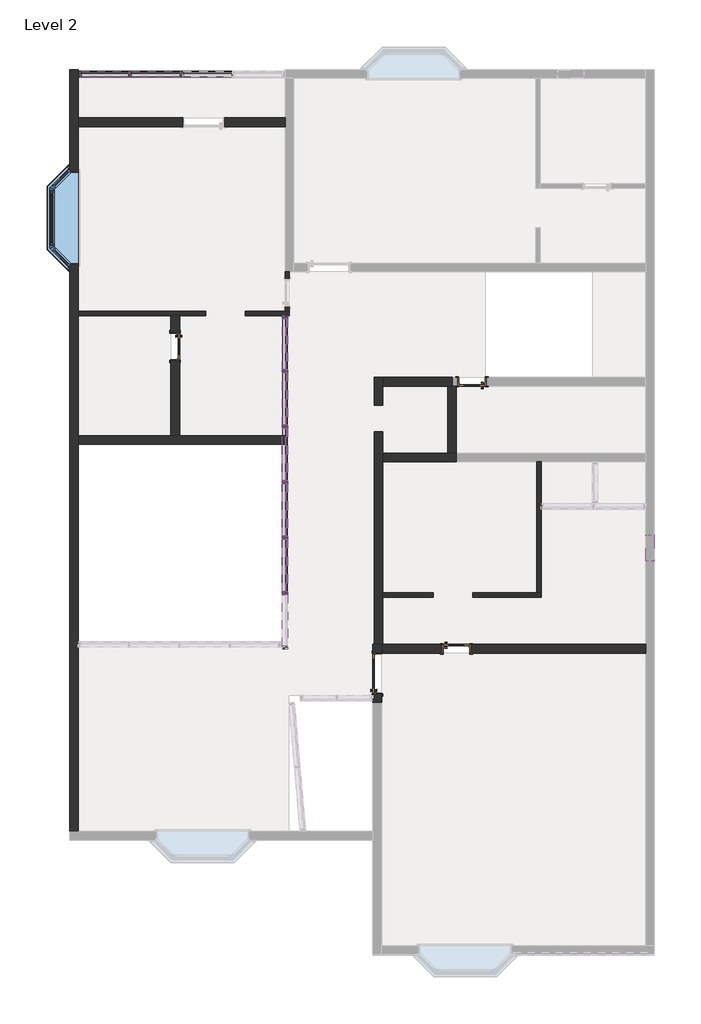
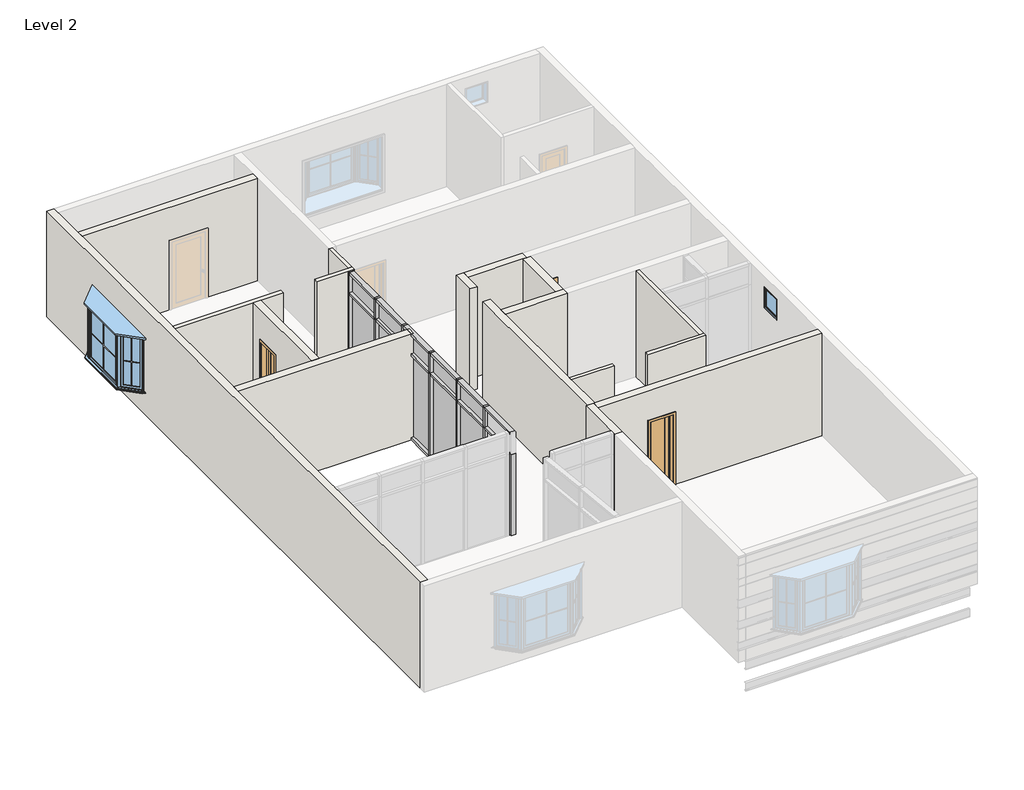
# One storey, part 4 of 5: 38 members, 17 walls, 12 plates, 4 doors, 2 windows.
"""IFC4 building model written with IfcOpenShell, lengths in millimetres."""

from ifc_helpers import new_model, si_unit, frame, origin, place, context, project, spatial, polyline, outline, extrude, faceted_brep, transform, mapped, element, save
from components import door_interior_single_1_panel_wood_5fe0af8f, door_interior_single_1_panel_wood_secondary_door_3_x_7_9c4ddfbd, member_6e77e263, member_47bfaf8a, member_f0fea5a5, member_ee409385, member_0e454ba5, member_3d117b0e, member_34cc32ae, member_667b8694, member_11eb1482, member_fb055d8d, member_66f4a397, member_e9262278, system_panel_glazed_d0e49211, system_panel_glazed_ecda40cd, system_panel_glazed_1bdee89b, system_panel_glazed_328a0544, system_panel_glazed_4fbe648e, system_panel_glazed_a20b732f, window_6846e476, window_9f89e8e4

model = new_model("IFC4")

# Units and contexts
model_context = context("Model", 3, world=origin())
ifc_project = project(units=[si_unit("LENGTHUNIT", "METRE", prefix="MILLI")], contexts=[model_context])

# Site, building, storey
site = spatial("IfcSite", under=ifc_project)
building = spatial("IfcBuilding", under=site)
storey = spatial("IfcBuildingStorey", under=building, Name="Level 2", Elevation=3048.0)

# Doors
placement = place(None, origin())
door_interior_single_1_panel_wood_shape = door_interior_single_1_panel_wood_5fe0af8f(model_context)
element("IfcDoor", 1, ObjectType="Door-Interior-Single-1_Panel-Wood", at=placement, inside=storey, context=model_context, shape_type="MappedRepresentation", body=[
    mapped(door_interior_single_1_panel_wood_shape, transform((-41818.5380314, -2936.7163973, 3048.0), x_axis=(1.0, 0.0, 0.0), y_axis=(0.0, 1.0, 0.0), z_axis=(0.0, 0.0, 1.0))),
])
element("IfcDoor", 2, ObjectType="Door-Interior-Single-1_Panel-Wood", at=placement, inside=storey, context=model_context, shape_type="MappedRepresentation", body=[
    mapped(door_interior_single_1_panel_wood_shape, transform((-41462.9380314, 3229.1336027, 3048.0), x_axis=(-1.0, 0.0, 0.0), y_axis=(0.0, -1.0, 0.0), z_axis=(0.0, 0.0, 1.0))),
])
element("IfcDoor", 3, ObjectType="Door-Interior-Single-1_Panel-Wood", at=placement, inside=storey, context=model_context, shape_type="MappedRepresentation", body=[
    mapped(door_interior_single_1_panel_wood_shape, transform((-48317.7630314, 4045.1086027, 3048.0), x_axis=(0.0, -1.0, 0.0), y_axis=(1.0, 0.0, 0.0), z_axis=(0.0, 0.0, 1.0))),
])
door_interior_single_1_panel_wood_secondary_door_3_x_7_shape = door_interior_single_1_panel_wood_secondary_door_3_x_7_9c4ddfbd(model_context)
element("IfcDoor", 4, ObjectType="Door-Interior-Single-1_Panel-Wood : SECONDARY DOOR 3' X 7'", at=placement, inside=storey, context=model_context, shape_type="MappedRepresentation", body=[
    mapped(door_interior_single_1_panel_wood_secondary_door_3_x_7_shape, transform((-43650.5130314, -3510.4922473, 3048.0), x_axis=(0.0, 1.0, 0.0), y_axis=(-1.0, 0.0, 0.0), z_axis=(0.0, 0.0, 1.0))),
])

# Members
member_shape = member_6e77e263(model_context)
element("IfcMember", 5, ObjectType="Rectangular Mullion : 2.5\" x 5\" rectangular", at=placement, inside=storey, context=model_context, shape_type="MappedRepresentation", body=[
    mapped(member_shape, transform((-45780.9380314, -1657.1913971, 5486.4), x_axis=(0.0, 1.0, 0.0), y_axis=(1.0, 0.0, 0.0), z_axis=(0.0, 0.0, -1.0))),
])
element("IfcMember", 6, ObjectType="Rectangular Mullion : 2.5\" x 5\" rectangular", at=placement, inside=storey, context=model_context, shape_type="MappedRepresentation", body=[
    mapped(member_shape, transform((-45780.9380314, -374.4913972, 5486.4), x_axis=(0.0, 1.0, 0.0), y_axis=(1.0, 0.0, 0.0), z_axis=(0.0, 0.0, -1.0))),
])
element("IfcMember", 7, ObjectType="Rectangular Mullion : 2.5\" x 5\" rectangular", at=placement, inside=storey, context=model_context, shape_type="MappedRepresentation", body=[
    mapped(member_shape, transform((-45780.9380314, 908.2086027, 5486.4), x_axis=(0.0, 1.0, 0.0), y_axis=(1.0, 0.0, 0.0), z_axis=(0.0, 0.0, -1.0))),
])
element("IfcMember", 8, ObjectType="Rectangular Mullion : 2.5\" x 5\" rectangular", at=placement, inside=storey, context=model_context, shape_type="MappedRepresentation", body=[
    mapped(member_shape, transform((-45780.9380314, 2190.9086026, 5486.4), x_axis=(0.0, 1.0, 0.0), y_axis=(1.0, 0.0, 0.0), z_axis=(0.0, 0.0, -1.0))),
])
element("IfcMember", 9, ObjectType="Rectangular Mullion : 2.5\" x 5\" rectangular", at=placement, inside=storey, context=model_context, shape_type="MappedRepresentation", body=[
    mapped(member_shape, transform((-45780.9380314, 3473.6086025, 5486.4), x_axis=(0.0, 1.0, 0.0), y_axis=(1.0, 0.0, 0.0), z_axis=(0.0, 0.0, -1.0))),
])
member_2_shape = member_47bfaf8a(model_context)
element("IfcMember", 10, ObjectType="Rectangular Mullion : 2.5\" x 5\" rectangular", at=placement, inside=storey, context=model_context, shape_type="MappedRepresentation", body=[
    mapped(member_2_shape, transform((-45780.9380314, 4756.3086027, 5486.4), x_axis=(0.0, 1.0, 0.0), y_axis=(1.0, 0.0, 0.0), z_axis=(0.0, 0.0, -1.0))),
])
member_3_shape = member_f0fea5a5(model_context)
element("IfcMember", 11, ObjectType="Rectangular Mullion : 2.5\" x 5\" rectangular", at=placement, inside=storey, context=model_context, shape_type="MappedRepresentation", body=[
    mapped(member_3_shape, transform((-45780.9380314, -1657.1913971, 3048.0), x_axis=(0.0, 1.0, 0.0), y_axis=(1.0, 0.0, 0.0), z_axis=(0.0, 0.0, -1.0))),
])
element("IfcMember", 12, ObjectType="Rectangular Mullion : 2.5\" x 5\" rectangular", at=placement, inside=storey, context=model_context, shape_type="MappedRepresentation", body=[
    mapped(member_3_shape, transform((-45780.9380314, -374.4913972, 3048.0), x_axis=(0.0, 1.0, 0.0), y_axis=(1.0, 0.0, 0.0), z_axis=(0.0, 0.0, -1.0))),
])
element("IfcMember", 13, ObjectType="Rectangular Mullion : 2.5\" x 5\" rectangular", at=placement, inside=storey, context=model_context, shape_type="MappedRepresentation", body=[
    mapped(member_3_shape, transform((-45780.9380314, 908.2086027, 3048.0), x_axis=(0.0, 1.0, 0.0), y_axis=(1.0, 0.0, 0.0), z_axis=(0.0, 0.0, -1.0))),
])
element("IfcMember", 14, ObjectType="Rectangular Mullion : 2.5\" x 5\" rectangular", at=placement, inside=storey, context=model_context, shape_type="MappedRepresentation", body=[
    mapped(member_3_shape, transform((-45780.9380314, 2190.9086026, 3048.0), x_axis=(0.0, 1.0, 0.0), y_axis=(1.0, 0.0, 0.0), z_axis=(0.0, 0.0, -1.0))),
])
element("IfcMember", 15, ObjectType="Rectangular Mullion : 2.5\" x 5\" rectangular", at=placement, inside=storey, context=model_context, shape_type="MappedRepresentation", body=[
    mapped(member_3_shape, transform((-45780.9380314, 3473.6086025, 3048.0), x_axis=(0.0, 1.0, 0.0), y_axis=(1.0, 0.0, 0.0), z_axis=(0.0, 0.0, -1.0))),
])
member_4_shape = member_ee409385(model_context)
element("IfcMember", 16, ObjectType="Rectangular Mullion : 2.5\" x 5\" rectangular", at=placement, inside=storey, context=model_context, shape_type="MappedRepresentation", body=[
    mapped(member_4_shape, transform((-45780.9380314, 4756.3086027, 3048.0), x_axis=(0.0, 1.0, 0.0), y_axis=(1.0, 0.0, 0.0), z_axis=(0.0, 0.0, -1.0))),
])
element("IfcMember", 17, ObjectType="Rectangular Mullion : 2.5\" x 5\" rectangular", at=placement, inside=storey, context=model_context, shape_type="MappedRepresentation", body=[
    mapped(member_4_shape, transform((-45780.9380314, -2939.8913973, 5486.4), x_axis=(0.0, -1.0, 0.0), y_axis=(1.0, 0.0, 0.0), z_axis=(0.0, 0.0, 1.0))),
])
member_5_shape = member_0e454ba5(model_context)
element("IfcMember", 18, ObjectType="Rectangular Mullion : 2.5\" x 5\" rectangular", at=placement, inside=storey, context=model_context, shape_type="MappedRepresentation", body=[
    mapped(member_5_shape, transform((-45780.9380314, 4692.8086027, 6096.0), x_axis=(0.0, 0.0, 1.0), y_axis=(1.0, 0.0, 0.0), z_axis=(0.0, 1.0, 0.0))),
])
element("IfcMember", 19, ObjectType="Rectangular Mullion : 2.5\" x 5\" rectangular", at=placement, inside=storey, context=model_context, shape_type="MappedRepresentation", body=[
    mapped(member_5_shape, transform((-45780.9380314, -1688.9413971, 6096.0), x_axis=(0.0, 0.0, 1.0), y_axis=(1.0, 0.0, 0.0), z_axis=(0.0, 1.0, 0.0))),
])
element("IfcMember", 20, ObjectType="Rectangular Mullion : 2.5\" x 5\" rectangular", at=placement, inside=storey, context=model_context, shape_type="MappedRepresentation", body=[
    mapped(member_5_shape, transform((-45780.9380314, 3505.3586025, 3048.0), x_axis=(0.0, 0.0, -1.0), y_axis=(1.0, 0.0, 0.0), z_axis=(0.0, -1.0, 0.0))),
])
member_6_shape = member_3d117b0e(model_context)
element("IfcMember", 21, ObjectType="Rectangular Mullion : 2.5\" x 5\" rectangular", at=placement, inside=storey, context=model_context, shape_type="MappedRepresentation", body=[
    mapped(member_6_shape, transform((-45780.9380314, -406.2413972, 6096.0), x_axis=(0.0, 0.0, 1.0), y_axis=(1.0, 0.0, 0.0), z_axis=(0.0, 1.0, 0.0))),
])
element("IfcMember", 22, ObjectType="Rectangular Mullion : 2.5\" x 5\" rectangular", at=placement, inside=storey, context=model_context, shape_type="MappedRepresentation", body=[
    mapped(member_6_shape, transform((-45780.9380314, 876.4586027, 6096.0), x_axis=(0.0, 0.0, 1.0), y_axis=(1.0, 0.0, 0.0), z_axis=(0.0, 1.0, 0.0))),
])
element("IfcMember", 23, ObjectType="Rectangular Mullion : 2.5\" x 5\" rectangular", at=placement, inside=storey, context=model_context, shape_type="MappedRepresentation", body=[
    mapped(member_6_shape, transform((-45780.9380314, 2159.1586026, 6096.0), x_axis=(0.0, 0.0, 1.0), y_axis=(1.0, 0.0, 0.0), z_axis=(0.0, 1.0, 0.0))),
])
element("IfcMember", 24, ObjectType="Rectangular Mullion : 2.5\" x 5\" rectangular", at=placement, inside=storey, context=model_context, shape_type="MappedRepresentation", body=[
    mapped(member_6_shape, transform((-45780.9380314, 3441.8586025, 6096.0), x_axis=(0.0, 0.0, 1.0), y_axis=(1.0, 0.0, 0.0), z_axis=(0.0, 1.0, 0.0))),
])
element("IfcMember", 25, ObjectType="Rectangular Mullion : 2.5\" x 5\" rectangular", at=placement, inside=storey, context=model_context, shape_type="MappedRepresentation", body=[
    mapped(member_6_shape, transform((-45780.9380314, -1625.4413971, 3048.0), x_axis=(0.0, 0.0, -1.0), y_axis=(1.0, 0.0, 0.0), z_axis=(0.0, -1.0, 0.0))),
])
element("IfcMember", 26, ObjectType="Rectangular Mullion : 2.5\" x 5\" rectangular", at=placement, inside=storey, context=model_context, shape_type="MappedRepresentation", body=[
    mapped(member_6_shape, transform((-45780.9380314, -342.7413972, 3048.0), x_axis=(0.0, 0.0, -1.0), y_axis=(1.0, 0.0, 0.0), z_axis=(0.0, -1.0, 0.0))),
])
element("IfcMember", 27, ObjectType="Rectangular Mullion : 2.5\" x 5\" rectangular", at=placement, inside=storey, context=model_context, shape_type="MappedRepresentation", body=[
    mapped(member_6_shape, transform((-45780.9380314, 939.9586027, 3048.0), x_axis=(0.0, 0.0, -1.0), y_axis=(1.0, 0.0, 0.0), z_axis=(0.0, -1.0, 0.0))),
])
element("IfcMember", 28, ObjectType="Rectangular Mullion : 2.5\" x 5\" rectangular", at=placement, inside=storey, context=model_context, shape_type="MappedRepresentation", body=[
    mapped(member_6_shape, transform((-45780.9380314, 2222.6586026, 3048.0), x_axis=(0.0, 0.0, -1.0), y_axis=(1.0, 0.0, 0.0), z_axis=(0.0, -1.0, 0.0))),
])
member_7_shape = member_34cc32ae(model_context)
element("IfcMember", 29, ObjectType="Rectangular Mullion : 2.5\" x 5\" rectangular", at=placement, inside=storey, context=model_context, shape_type="MappedRepresentation", body=[
    mapped(member_7_shape, transform((-45780.9380314, -1688.9413971, 5486.4), x_axis=(0.0, 0.0, 1.0), y_axis=(1.0, 0.0, 0.0), z_axis=(0.0, 1.0, 0.0))),
])
element("IfcMember", 30, ObjectType="Rectangular Mullion : 2.5\" x 5\" rectangular", at=placement, inside=storey, context=model_context, shape_type="MappedRepresentation", body=[
    mapped(member_7_shape, transform((-45780.9380314, 4692.8086027, 5486.4), x_axis=(0.0, 0.0, 1.0), y_axis=(1.0, 0.0, 0.0), z_axis=(0.0, 1.0, 0.0))),
])
member_8_shape = member_667b8694(model_context)
element("IfcMember", 31, ObjectType="Rectangular Mullion : 2.5\" x 5\" rectangular", at=placement, inside=storey, context=model_context, shape_type="MappedRepresentation", body=[
    mapped(member_8_shape, transform((-45780.9380314, -406.2413972, 5486.4), x_axis=(0.0, 0.0, 1.0), y_axis=(1.0, 0.0, 0.0), z_axis=(0.0, 1.0, 0.0))),
])
element("IfcMember", 32, ObjectType="Rectangular Mullion : 2.5\" x 5\" rectangular", at=placement, inside=storey, context=model_context, shape_type="MappedRepresentation", body=[
    mapped(member_8_shape, transform((-45780.9380314, 876.4586027, 5486.4), x_axis=(0.0, 0.0, 1.0), y_axis=(1.0, 0.0, 0.0), z_axis=(0.0, 1.0, 0.0))),
])
element("IfcMember", 33, ObjectType="Rectangular Mullion : 2.5\" x 5\" rectangular", at=placement, inside=storey, context=model_context, shape_type="MappedRepresentation", body=[
    mapped(member_8_shape, transform((-45780.9380314, 2159.1586026, 5486.4), x_axis=(0.0, 0.0, 1.0), y_axis=(1.0, 0.0, 0.0), z_axis=(0.0, 1.0, 0.0))),
])
element("IfcMember", 34, ObjectType="Rectangular Mullion : 2.5\" x 5\" rectangular", at=placement, inside=storey, context=model_context, shape_type="MappedRepresentation", body=[
    mapped(member_8_shape, transform((-45780.9380314, 3441.8586025, 5486.4), x_axis=(0.0, 0.0, 1.0), y_axis=(1.0, 0.0, 0.0), z_axis=(0.0, 1.0, 0.0))),
])
member_9_shape = member_11eb1482(model_context)
element("IfcMember", 35, ObjectType="Rectangular Mullion : 2.5\" x 5\" rectangular", at=placement, inside=storey, context=model_context, shape_type="MappedRepresentation", body=[
    mapped(member_9_shape, transform((-49394.0880313, 10344.3086027, 5209.4673659), x_axis=(0.0, 0.0, 1.0), y_axis=(0.0, -1.0, 0.0), z_axis=(1.0, 0.0, 0.0))),
])
member_10_shape = member_fb055d8d(model_context)
element("IfcMember", 36, ObjectType="Rectangular Mullion : 2.5\" x 5\" rectangular", at=placement, inside=storey, context=model_context, shape_type="MappedRepresentation", body=[
    mapped(member_10_shape, transform((-48200.2880314, 10344.3086027, 5209.4673659), x_axis=(0.0, 0.0, 1.0), y_axis=(0.0, -1.0, 0.0), z_axis=(1.0, 0.0, 0.0))),
])
element("IfcMember", 37, ObjectType="Rectangular Mullion : 2.5\" x 5\" rectangular", at=placement, inside=storey, context=model_context, shape_type="MappedRepresentation", body=[
    mapped(member_9_shape, transform((-50492.6380314, 10344.3086027, 3048.0), x_axis=(0.0, 0.0, -1.0), y_axis=(0.0, -1.0, 0.0), z_axis=(-1.0, 0.0, 0.0))),
])
element("IfcMember", 38, ObjectType="Rectangular Mullion : 2.5\" x 5\" rectangular", at=placement, inside=storey, context=model_context, shape_type="MappedRepresentation", body=[
    mapped(member_10_shape, transform((-49330.5880313, 10344.3086027, 3048.0), x_axis=(0.0, 0.0, -1.0), y_axis=(0.0, -1.0, 0.0), z_axis=(-1.0, 0.0, 0.0))),
])
element("IfcMember", 39, ObjectType="Rectangular Mullion : 2.5\" x 5\" rectangular", at=placement, inside=storey, context=model_context, shape_type="MappedRepresentation", body=[
    mapped(member_10_shape, transform((-48136.7880314, 10344.3086027, 3048.0), x_axis=(0.0, 0.0, -1.0), y_axis=(0.0, -1.0, 0.0), z_axis=(-1.0, 0.0, 0.0))),
])
member_11_shape = member_66f4a397(model_context)
element("IfcMember", 40, ObjectType="Rectangular Mullion : 2.5\" x 5\" rectangular", at=placement, inside=storey, context=model_context, shape_type="MappedRepresentation", body=[
    mapped(member_11_shape, transform((-49362.3380313, 10344.3086027, 3048.0), x_axis=(1.0, 0.0, 0.0), y_axis=(0.0, -1.0, 0.0), z_axis=(0.0, 0.0, -1.0))),
])
element("IfcMember", 41, ObjectType="Rectangular Mullion : 2.5\" x 5\" rectangular", at=placement, inside=storey, context=model_context, shape_type="MappedRepresentation", body=[
    mapped(member_11_shape, transform((-48168.5380314, 10344.3086027, 3048.0), x_axis=(1.0, 0.0, 0.0), y_axis=(0.0, -1.0, 0.0), z_axis=(0.0, 0.0, -1.0))),
])
member_12_shape = member_e9262278(model_context)
element("IfcMember", 42, ObjectType="Rectangular Mullion : 2.5\" x 5\" rectangular", at=placement, inside=storey, context=model_context, shape_type="MappedRepresentation", body=[
    mapped(member_12_shape, transform((-50556.1380314, 10344.3086027, 5209.4673659), x_axis=(-1.0, 0.0, 0.0), y_axis=(0.0, -1.0, 0.0), z_axis=(0.0, 0.0, 1.0))),
])

# Plates
system_panel_glazed_shape = system_panel_glazed_d0e49211(model_context)
element("IfcPlate", 43, ObjectType="System Panel : Glazed", at=placement, inside=storey, context=model_context, shape_type="MappedRepresentation", body=[
    mapped(system_panel_glazed_shape, transform((-45780.9380314, 4099.0836026, 3111.5), x_axis=(0.0, 1.0, 0.0), y_axis=(-1.0, 0.0, 0.0), z_axis=(0.0, 0.0, 1.0))),
])
system_panel_glazed_2_shape = system_panel_glazed_ecda40cd(model_context)
element("IfcPlate", 44, ObjectType="System Panel : Glazed", at=placement, inside=storey, context=model_context, shape_type="MappedRepresentation", body=[
    mapped(system_panel_glazed_2_shape, transform((-45780.9380314, -1015.8413971, 3111.5), x_axis=(0.0, 1.0, 0.0), y_axis=(-1.0, 0.0, 0.0), z_axis=(0.0, 0.0, 1.0))),
])
element("IfcPlate", 45, ObjectType="System Panel : Glazed", at=placement, inside=storey, context=model_context, shape_type="MappedRepresentation", body=[
    mapped(system_panel_glazed_2_shape, transform((-45780.9380314, 266.8586028, 3111.5), x_axis=(0.0, 1.0, 0.0), y_axis=(-1.0, 0.0, 0.0), z_axis=(0.0, 0.0, 1.0))),
])
element("IfcPlate", 46, ObjectType="System Panel : Glazed", at=placement, inside=storey, context=model_context, shape_type="MappedRepresentation", body=[
    mapped(system_panel_glazed_2_shape, transform((-45780.9380314, 1549.5586027, 3111.5), x_axis=(0.0, 1.0, 0.0), y_axis=(-1.0, 0.0, 0.0), z_axis=(0.0, 0.0, 1.0))),
])
element("IfcPlate", 47, ObjectType="System Panel : Glazed", at=placement, inside=storey, context=model_context, shape_type="MappedRepresentation", body=[
    mapped(system_panel_glazed_2_shape, transform((-45780.9380314, 2832.2586026, 3111.5), x_axis=(0.0, 1.0, 0.0), y_axis=(-1.0, 0.0, 0.0), z_axis=(0.0, 0.0, 1.0))),
])
system_panel_glazed_3_shape = system_panel_glazed_1bdee89b(model_context)
element("IfcPlate", 48, ObjectType="System Panel : Glazed", at=placement, inside=storey, context=model_context, shape_type="MappedRepresentation", body=[
    mapped(system_panel_glazed_3_shape, transform((-45780.9380314, 4099.0836026, 5518.15), x_axis=(0.0, 1.0, 0.0), y_axis=(-1.0, 0.0, 0.0), z_axis=(0.0, 0.0, 1.0))),
])
system_panel_glazed_4_shape = system_panel_glazed_328a0544(model_context)
element("IfcPlate", 49, ObjectType="System Panel : Glazed", at=placement, inside=storey, context=model_context, shape_type="MappedRepresentation", body=[
    mapped(system_panel_glazed_4_shape, transform((-45780.9380314, -1015.8413971, 5518.15), x_axis=(0.0, 1.0, 0.0), y_axis=(-1.0, 0.0, 0.0), z_axis=(0.0, 0.0, 1.0))),
])
element("IfcPlate", 50, ObjectType="System Panel : Glazed", at=placement, inside=storey, context=model_context, shape_type="MappedRepresentation", body=[
    mapped(system_panel_glazed_4_shape, transform((-45780.9380314, 266.8586028, 5518.15), x_axis=(0.0, 1.0, 0.0), y_axis=(-1.0, 0.0, 0.0), z_axis=(0.0, 0.0, 1.0))),
])
element("IfcPlate", 51, ObjectType="System Panel : Glazed", at=placement, inside=storey, context=model_context, shape_type="MappedRepresentation", body=[
    mapped(system_panel_glazed_4_shape, transform((-45780.9380314, 1549.5586027, 5518.15), x_axis=(0.0, 1.0, 0.0), y_axis=(-1.0, 0.0, 0.0), z_axis=(0.0, 0.0, 1.0))),
])
element("IfcPlate", 52, ObjectType="System Panel : Glazed", at=placement, inside=storey, context=model_context, shape_type="MappedRepresentation", body=[
    mapped(system_panel_glazed_4_shape, transform((-45780.9380314, 2832.2586026, 5518.15), x_axis=(0.0, 1.0, 0.0), y_axis=(-1.0, 0.0, 0.0), z_axis=(0.0, 0.0, 1.0))),
])
system_panel_glazed_5_shape = system_panel_glazed_4fbe648e(model_context)
element("IfcPlate", 53, ObjectType="System Panel : Glazed", at=placement, inside=storey, context=model_context, shape_type="MappedRepresentation", body=[
    mapped(system_panel_glazed_5_shape, transform((-49943.3630313, 10344.3086027, 3111.5), x_axis=(1.0, 0.0, 0.0), y_axis=(0.0, 1.0, 0.0), z_axis=(0.0, 0.0, 1.0))),
])
system_panel_glazed_6_shape = system_panel_glazed_a20b732f(model_context)
element("IfcPlate", 54, ObjectType="System Panel : Glazed", at=placement, inside=storey, context=model_context, shape_type="MappedRepresentation", body=[
    mapped(system_panel_glazed_6_shape, transform((-48765.4380313, 10344.3086027, 3111.5), x_axis=(1.0, 0.0, 0.0), y_axis=(0.0, 1.0, 0.0), z_axis=(0.0, 0.0, 1.0))),
])

# Walls
element("IfcWall", 55, ObjectType="INNER WALL 4\"", at=placement, inside=storey, context=model_context, shape_type="SweptSolid", body=[
    extrude(outline(polyline([(-42351.9380314, -1746.0913973), (-43520.3380314, -1746.0913973), (-43520.3380314, -1644.4913973), (-42351.9380314, -1644.4913973), (-42351.9380314, -1746.0913973)])), frame((0.0, 0.0, 3048.0), z_axis=(0.0, 0.0, 1.0), x_axis=(1.0, 0.0, 0.0)), (0.0, 0.0, 1.0), 3048.0),
])
element("IfcWall", 56, ObjectType="INNER WALL 4\"", at=placement, inside=storey, context=model_context, shape_type="Brep", body=[
    faceted_brep([(-41437.5380314, -1746.0913973, 3048.0), (-39862.7380314, -1746.0913973, 3048.0), (-39862.7380314, -1746.0913973, 6096.0), (-41437.5380314, -1746.0913973, 6096.0), (-41437.5380314, -1644.4913973, 3048.0), (-41437.5380314, -1644.4913973, 6096.0), (-39964.3380314, -1644.4913973, 6096.0), (-39862.7380314, -1644.4913973, 6096.0), (-39862.7380314, -1644.4913973, 3048.0), (-39964.3380314, -1644.4913973, 3048.0)], [[[0, 1, 2, 3]], [[4, 5, 6, 7, 8, 9]], [[1, 0, 4, 9, 8]], [[3, 2, 7, 6, 5]], [[0, 3, 5, 4]], [[2, 1, 8, 7]]]),
])
element("IfcWall", 57, ObjectType="INNER WALL 4\"", at=placement, inside=storey, context=model_context, shape_type="Brep", body=[
    faceted_brep([(-39862.7380314, -1644.4913973, 3048.0), (-39862.7380314, 303.5957124, 3048.0), (-39862.7380314, 354.3957124, 3048.0), (-39862.7380314, 1378.1086027, 3048.0), (-39862.7380314, 1378.1086027, 6096.0), (-39862.7380314, 354.3957124, 6096.0), (-39862.7380314, 303.5957124, 6096.0), (-39862.7380314, -1644.4913973, 6096.0), (-39964.3380314, -1644.4913973, 3048.0), (-39964.3380314, -1644.4913973, 6096.0), (-39964.3380314, 1378.1086027, 6096.0), (-39964.3380314, 1378.1086027, 3048.0)], [[[0, 1, 2, 3, 4, 5, 6, 7]], [[8, 9, 10, 11]], [[3, 2, 1, 0, 8, 11]], [[7, 6, 5, 4, 10, 9]], [[0, 7, 9, 8]], [[4, 3, 11, 10]]]),
])
element("IfcWall", 58, ObjectType="INNER WALL 4\"", at=placement, inside=storey, context=model_context, shape_type="Brep", body=[
    faceted_brep([(-50556.1380314, 4756.3086027, 3048.0), (-48422.5380314, 4756.3086027, 3048.0), (-48219.3380314, 4756.3086027, 3048.0), (-47609.7380314, 4756.3086027, 3048.0), (-47609.7380314, 4756.3086027, 6096.0), (-48219.3380314, 4756.3086027, 6096.0), (-48422.5380314, 4756.3086027, 6096.0), (-50556.1380314, 4756.3086027, 6096.0), (-50556.1380314, 4857.9086027, 3048.0), (-50556.1380314, 4857.9086027, 6096.0), (-47609.7380314, 4857.9086027, 6096.0), (-47609.7380314, 4857.9086027, 3048.0)], [[[0, 1, 2, 3, 4, 5, 6, 7]], [[8, 9, 10, 11]], [[3, 2, 1, 0, 8, 11]], [[4, 3, 11, 10]], [[7, 6, 5, 4, 10, 9]], [[0, 7, 9, 8]]]),
])
element("IfcWall", 59, ObjectType="INNER WALL 4\"", at=placement, inside=storey, context=model_context, shape_type="Brep", body=[
    faceted_brep([(-46695.3380314, 4756.3086027, 3048.0), (-45679.3380314, 4756.3086027, 3048.0), (-45679.3380314, 4756.3086027, 6096.0), (-46695.3380314, 4756.3086027, 6096.0), (-46695.3380314, 4857.9086027, 3048.0), (-46695.3380314, 4857.9086027, 6096.0), (-45780.9380314, 4857.9086027, 6096.0), (-45679.3380314, 4857.9086027, 6096.0), (-45679.3380314, 4857.9086027, 3048.0), (-45780.9380314, 4857.9086027, 3048.0)], [[[0, 1, 2, 3]], [[4, 5, 6, 7, 8, 9]], [[1, 0, 4, 9, 8]], [[3, 2, 7, 6, 5]], [[0, 3, 5, 4]], [[2, 1, 8, 7]]]),
])
element("IfcWall", 60, ObjectType="INNER WALL 4\"", at=placement, inside=storey, context=model_context, shape_type="SweptSolid", body=[
    extrude(outline(polyline([(4857.9086027, 6096.0), (5772.3086027, 6096.0), (5772.3086027, 3048.0), (5619.9086027, 3048.0), (5619.9086027, 5207.0), (4959.5086027, 5207.0), (4959.5086027, 3048.0), (4857.9086027, 3048.0), (4857.9086027, 6096.0)])), frame((-45780.9380314, 0.0, 0.0), z_axis=(1.0, 0.0, 0.0), x_axis=(0.0, 1.0, 0.0)), (0.0, 0.0, 1.0), 101.6),
])
element("IfcWall", 61, ObjectType="OUTER WALL 8\"", at=placement, inside=storey, context=model_context, shape_type="Brep", body=[
    faceted_brep([(-50759.3380314, 10445.9086027, 3048.0), (-50759.3380314, -7156.2913973, 3048.0), (-50759.3380314, -7156.2913973, 6096.0), (-50759.3380314, 10445.9086027, 6096.0), (-50759.3380314, 8133.1000114, 5232.4), (-50759.3380314, 5900.7171941, 5232.4), (-50759.3380314, 5900.7171941, 3657.6), (-50759.3380314, 8133.1000114, 3657.6), (-50556.1380314, 10445.9086027, 3048.0), (-50556.1380314, 10445.9086027, 5209.4673659), (-50556.1380314, 10445.9086027, 6096.0), (-50556.1380314, 10242.7086027, 6096.0), (-50556.1380314, 9328.3086027, 6096.0), (-50556.1380314, 9125.1086027, 6096.0), (-50556.1380314, 4857.9086027, 6096.0), (-50556.1380314, 4756.3086027, 6096.0), (-50556.1380314, 1987.7086027, 6096.0), (-50556.1380314, 1784.5086027, 6096.0), (-50556.1380314, -7156.2913973, 6096.0), (-50556.1380314, -7156.2913973, 3048.0), (-50556.1380314, 1784.5086027, 3048.0), (-50556.1380314, 1987.7086027, 3048.0), (-50556.1380314, 4756.3086027, 3048.0), (-50556.1380314, 4857.9086027, 3048.0), (-50556.1380314, 9125.1086027, 3048.0), (-50556.1380314, 9328.3086027, 3048.0), (-50556.1380314, 5950.1086027, 5232.4), (-50556.1380314, 8083.7086027, 5232.4), (-50556.1380314, 8083.7086027, 3657.6), (-50556.1380314, 5950.1086027, 3657.6), (-50709.9466227, 5950.1086027, 5232.4), (-50709.9466227, 8083.7086027, 5232.4), (-50709.9466227, 5950.1086027, 3657.6), (-50709.9466227, 8083.7086027, 3657.6)], [[[0, 1, 2, 3], [4, 5, 6, 7]], [[8, 9, 10, 11, 12, 13, 14, 15, 16, 17, 18, 19, 20, 21, 22, 23, 24, 25], [26, 27, 28, 29]], [[1, 0, 8, 25, 24, 23, 22, 21, 20, 19]], [[3, 2, 18, 17, 16, 15, 14, 13, 12, 11, 10]], [[2, 1, 19, 18]], [[0, 3, 10, 9, 8]], [[30, 5, 4, 31, 27, 26]], [[32, 29, 28, 33, 7, 6]], [[30, 26, 29, 32]], [[27, 31, 33, 28]], [[31, 4, 7, 33]], [[5, 30, 32, 6]]]),
])
element("IfcWall", 62, ObjectType="OUTER WALL 8\"", at=placement, inside=storey, context=model_context, shape_type="Brep", body=[
    faceted_brep([(-50556.1380314, 1784.5086027, 3048.0), (-45780.9380314, 1784.5086027, 3048.0), (-45780.9380314, 1784.5086027, 6096.0), (-50556.1380314, 1784.5086027, 6096.0), (-50556.1380314, 1987.7086027, 3048.0), (-50556.1380314, 1987.7086027, 6096.0), (-48422.5380314, 1987.7086027, 6096.0), (-48219.3380314, 1987.7086027, 6096.0), (-45780.9380314, 1987.7086027, 6096.0), (-45780.9380314, 1987.7086027, 3048.0), (-48219.3380314, 1987.7086027, 3048.0), (-48422.5380314, 1987.7086027, 3048.0)], [[[0, 1, 2, 3]], [[4, 5, 6, 7, 8, 9, 10, 11]], [[1, 0, 4, 11, 10, 9]], [[2, 1, 9, 8]], [[3, 2, 8, 7, 6, 5]], [[0, 3, 5, 4]]]),
])
element("IfcWall", 63, ObjectType="OUTER WALL 8\"", at=placement, inside=storey, context=model_context, shape_type="SweptSolid", body=[
    extrude(outline(polyline([(1987.7086027, 6096.0), (4756.3086027, 6096.0), (4756.3086027, 3048.0), (4375.3086027, 3048.0), (4375.3086027, 5207.0), (3714.9086027, 5207.0), (3714.9086027, 3048.0), (1987.7086027, 3048.0), (1987.7086027, 6096.0)])), frame((-48422.5380314, 0.0, 0.0), z_axis=(1.0, 0.0, 0.0), x_axis=(0.0, 1.0, 0.0)), (0.0, 0.0, 1.0), 203.2),
])
element("IfcWall", 64, ObjectType="OUTER WALL 8\"", at=placement, inside=storey, context=model_context, shape_type="Brep", body=[
    faceted_brep([(-43545.7380314, -2838.2913973, 6096.0), (-43545.7380314, -3041.4913973, 6096.0), (-43545.7380314, -4182.6930974, 6096.0), (-43545.7380314, -4182.6930974, 3048.0), (-43545.7380314, -3993.0922473, 3048.0), (-43545.7380314, -3993.0922473, 5207.0), (-43545.7380314, -3027.8922473, 5207.0), (-43545.7380314, -3027.8922473, 3048.0), (-43545.7380314, -2838.2913973, 3048.0), (-43748.9380314, -4182.6930974, 6096.0), (-43748.9380314, -2838.2913973, 6096.0), (-43748.9380314, -2838.2913973, 3048.0), (-43748.9380314, -3027.8922473, 3048.0), (-43748.9380314, -3027.8922473, 5207.0), (-43748.9380314, -3993.0922473, 5207.0), (-43748.9380314, -3993.0922473, 3048.0), (-43748.9380314, -4182.6930974, 3048.0), (-43723.5380314, -2838.2913973, 3048.0), (-43723.5380314, -2838.2913973, 6096.0)], [[[0, 1, 2, 3, 4, 5, 6, 7, 8]], [[9, 10, 11, 12, 13, 14, 15, 16]], [[11, 17, 8, 7, 12]], [[3, 16, 15, 4]], [[2, 1, 0, 18, 10, 9]], [[3, 2, 9, 16]], [[0, 8, 17, 11, 10, 18]], [[6, 13, 12, 7]], [[13, 6, 5, 14]], [[14, 5, 4, 15]]]),
])
element("IfcWall", 65, ObjectType="OUTER WALL 8\"", at=placement, inside=storey, context=model_context, shape_type="Brep", body=[
    faceted_brep([(-43545.7380314, -2838.2913973, 6096.0), (-43520.3380314, -2838.2913973, 6096.0), (-37449.7380314, -2838.2913973, 6096.0), (-37449.7380314, -2838.2913973, 3048.0), (-41488.3380314, -2838.2913973, 3048.0), (-41488.3380314, -2838.2913973, 5207.0), (-42148.7380314, -2838.2913973, 5207.0), (-42148.7380314, -2838.2913973, 3048.0), (-43520.3380314, -2838.2913973, 3048.0), (-43545.7380314, -2838.2913973, 3048.0), (-37449.7380314, -3041.4913973, 6096.0), (-43545.7380314, -3041.4913973, 6096.0), (-43545.7380314, -3041.4913973, 3048.0), (-42148.7380314, -3041.4913973, 3048.0), (-42148.7380314, -3041.4913973, 5207.0), (-41488.3380314, -3041.4913973, 5207.0), (-41488.3380314, -3041.4913973, 3048.0), (-37449.7380314, -3041.4913973, 3048.0)], [[[0, 1, 2, 3, 4, 5, 6, 7, 8, 9]], [[10, 11, 12, 13, 14, 15, 16, 17]], [[3, 17, 16, 4]], [[12, 9, 8, 7, 13]], [[2, 1, 0, 11, 10]], [[0, 9, 12, 11]], [[3, 2, 10, 17]], [[15, 5, 4, 16]], [[5, 15, 14, 6]], [[6, 14, 13, 7]]]),
])
element("IfcWall", 66, ObjectType="OUTER WALL 8\"", at=placement, inside=storey, context=model_context, shape_type="Brep", body=[
    faceted_brep([(-43520.3380314, -2838.2913973, 3048.0), (-43520.3380314, -1746.0913973, 3048.0), (-43520.3380314, -1644.4913973, 3048.0), (-43520.3380314, 1378.1086027, 3048.0), (-43520.3380314, 1581.3086027, 3048.0), (-43520.3380314, 2076.6086027, 3048.0), (-43520.3380314, 2076.6086027, 6096.0), (-43520.3380314, 1581.3086027, 6096.0), (-43520.3380314, 1378.1086027, 6096.0), (-43520.3380314, -1644.4913973, 6096.0), (-43520.3380314, -1746.0913973, 6096.0), (-43520.3380314, -2838.2913973, 6096.0), (-43723.5380314, -2838.2913973, 3048.0), (-43723.5380314, -2838.2913973, 6096.0), (-43723.5380314, 2076.6086027, 6096.0), (-43723.5380314, 2076.6086027, 3048.0), (-43545.7380314, -2838.2913973, 3048.0), (-43545.7380314, -2838.2913973, 6096.0)], [[[0, 1, 2, 3, 4, 5, 6, 7, 8, 9, 10, 11]], [[12, 13, 14, 15]], [[5, 4, 3, 2, 1, 0, 16, 12, 15]], [[6, 5, 15, 14]], [[11, 10, 9, 8, 7, 6, 14, 13, 17]], [[0, 11, 17, 13, 12, 16]]]),
])
element("IfcWall", 67, ObjectType="OUTER WALL 8\"", at=placement, inside=storey, context=model_context, shape_type="SweptSolid", body=[
    extrude(outline(polyline([(6096.0, -45780.9380314), (6096.0, -50556.1380314), (3048.0, -50556.1380314), (3048.0, -48143.1380314), (5105.4, -48143.1380314), (5105.4, -47177.9380314), (3048.0, -47177.9380314), (3048.0, -45780.9380314), (6096.0, -45780.9380314)])), frame((0.0, 9125.1086027, 0.0), z_axis=(0.0, 1.0, 0.0), x_axis=(0.0, 0.0, 1.0)), (0.0, 0.0, 1.0), 203.2),
])
element("IfcWall", 68, ObjectType="OUTER WALL 8\"", at=placement, inside=storey, context=model_context, shape_type="Brep", body=[
    faceted_brep([(-43520.3380314, 2686.2086027, 3048.0), (-43520.3380314, 3130.7086027, 3048.0), (-43520.3380314, 3333.9086027, 3048.0), (-43520.3380314, 3333.9086027, 6096.0), (-43520.3380314, 3130.7086027, 6096.0), (-43520.3380314, 2686.2086027, 6096.0), (-43723.5380314, 2686.2086027, 3048.0), (-43723.5380314, 2686.2086027, 6096.0), (-43723.5380314, 3333.9086027, 6096.0), (-43723.5380314, 3333.9086027, 3048.0)], [[[0, 1, 2, 3, 4, 5]], [[6, 7, 8, 9]], [[2, 1, 0, 6, 9]], [[5, 4, 3, 8, 7]], [[0, 5, 7, 6]], [[3, 2, 9, 8]]]),
])
element("IfcWall", 69, ObjectType="OUTER WALL 8\"", at=placement, inside=storey, context=model_context, shape_type="Brep", body=[
    faceted_brep([(-43520.3380314, 3130.7086027, 3048.0), (-42021.7380314, 3130.7086027, 3048.0), (-41920.1380314, 3130.7086027, 3048.0), (-41920.1380314, 3130.7086027, 6096.0), (-42021.7380314, 3130.7086027, 6096.0), (-43520.3380314, 3130.7086027, 6096.0), (-43520.3380314, 3333.9086027, 3048.0), (-43520.3380314, 3333.9086027, 6096.0), (-41920.1380314, 3333.9086027, 6096.0), (-41920.1380314, 3333.9086027, 3048.0)], [[[0, 1, 2, 3, 4, 5]], [[6, 7, 8, 9]], [[2, 1, 0, 6, 9]], [[3, 2, 9, 8]], [[5, 4, 3, 8, 7]], [[0, 5, 7, 6]]]),
])
element("IfcWall", 70, ObjectType="OUTER WALL 8\"", at=placement, inside=storey, context=model_context, shape_type="Brep", body=[
    faceted_brep([(-43520.3380314, 1378.1086027, 3048.0), (-41818.5380314, 1378.1086027, 3048.0), (-41818.5380314, 1378.1086027, 6096.0), (-43520.3380314, 1378.1086027, 6096.0), (-43520.3380314, 1581.3086027, 3048.0), (-43520.3380314, 1581.3086027, 6096.0), (-42021.7380314, 1581.3086027, 6096.0), (-41818.5380314, 1581.3086027, 6096.0), (-41818.5380314, 1581.3086027, 3048.0), (-42021.7380314, 1581.3086027, 3048.0)], [[[0, 1, 2, 3]], [[4, 5, 6, 7, 8, 9]], [[1, 0, 4, 9, 8]], [[3, 2, 7, 6, 5]], [[0, 3, 5, 4]], [[2, 1, 8, 7]]]),
])
element("IfcWall", 71, ObjectType="OUTER WALL 8\"", at=placement, inside=storey, context=model_context, shape_type="Brep", body=[
    faceted_brep([(-41818.5380314, 1581.3086027, 3048.0), (-41818.5380314, 3130.7086027, 3048.0), (-41818.5380314, 3130.7086027, 6096.0), (-41818.5380314, 1581.3086027, 6096.0), (-42021.7380314, 1581.3086027, 3048.0), (-42021.7380314, 1581.3086027, 6096.0), (-42021.7380314, 3130.7086027, 6096.0), (-42021.7380314, 3130.7086027, 3048.0), (-41920.1380314, 3130.7086027, 3048.0), (-41920.1380314, 3130.7086027, 6096.0)], [[[0, 1, 2, 3]], [[4, 5, 6, 7]], [[1, 0, 4, 7, 8]], [[3, 2, 9, 6, 5]], [[0, 3, 5, 4]], [[2, 1, 8, 7, 6, 9]]]),
])

# Windows
window_shape = window_6846e476(model_context)
element("IfcWindow", 72, ObjectType="Fixed : 24\" x 24\"", at=placement, inside=storey, context=model_context, shape_type="MappedRepresentation", body=[
    mapped(window_shape, transform((-37348.1380314, -572.7042876, 4267.2), x_axis=(0.0, 1.0, 0.0), y_axis=(-1.0, 0.0, 0.0), z_axis=(0.0, 0.0, 1.0))),
])
window_2_shape = window_9f89e8e4(model_context)
element("IfcWindow", 73, ObjectType="Window-Bay-Casement-45_Degree_Angle : 84\" x 60\" x 18\"", at=placement, inside=storey, context=model_context, shape_type="MappedRepresentation", body=[
    mapped(window_2_shape, transform((-50657.7380314, 7016.9086027, 3048.0), x_axis=(0.0, 1.0, 0.0), y_axis=(-1.0, 0.0, 0.0), z_axis=(0.0, 0.0, 1.0))),
])

save(model, "model.ifc")

# Revit data of these elements
# Type "Door-Interior-Single-1_Panel-Wood"
#   Type Mark = "12"
#   Assembly Code = "C1020300"
#   Analytic Construction = "Wooden"
#   Top Rail = 0' - 4 11/16"
#   Thickness = 0' - 1 3/8"
#   Thermal Resistance (R) = 2.5876 (h·ft²·°F)/BTU
#   Swing Angle [instance default] = 90.00°
#   Stiles = 0' - 4 3/4"
#   Rough Width = 2' - 2"
#   Rough Height = 7' - 1"
#   Height = 7' - 0"
#   Width = 2' - 0"
#   Heat Transfer Coefficient (U) = 0.3865 BTU/(h·ft²·°F)
#   Bottom Rail = 0' - 9 1/8"
#   Trim Material = Cherry
#   Panel Material = Cherry
#   Frame Material = Cherry
#   Door Handle Material = Aluminum
#   Visual Light Transmittance = 0
#   Solar Heat Gain Coefficient = 0
#   Wall Closure = (empty or 0)
#   Function = (empty or 0)
# Type "Door-Interior-Single-1_Panel-Wood : SECONDARY DOOR 3' X 7'"
#   Type Mark = "11"
#   Assembly Code = "C1020300"
#   Analytic Construction = "Wooden"
#   Top Rail = 0' - 4 11/16"
#   Thickness = 0' - 1 3/8"
#   Thermal Resistance (R) = 2.5876 (h·ft²·°F)/BTU
#   Swing Angle [instance default] = 90.00°
#   Stiles = 0' - 4 3/4"
#   Rough Width = 3' - 2"
#   Rough Height = 7' - 1"
#   Height = 7' - 0"
#   Width = 3' - 0"
#   Heat Transfer Coefficient (U) = 0.3865 BTU/(h·ft²·°F)
#   Bottom Rail = 0' - 9 1/8"
#   Trim Material = Cherry
#   Panel Material = Cherry
#   Frame Material = Cherry
#   Door Handle Material = Aluminum
#   Visual Light Transmittance = 0
#   Solar Heat Gain Coefficient = 0
#   Wall Closure = (empty or 0)
#   Function = (empty or 0)
# Type "Rectangular Mullion : 2.5\" x 5\" rectangular"
#   built-in parameter 1007304 = 0.416667 (stored number, unit not read)
#   built-in parameter 1007301 = 0.104167 (stored number, unit not read)
#   built-in parameter 1007300 = 0.104167 (stored number, unit not read)
# Type "System Panel : Glazed"
#   Construction Type Id = "GSP4R"
#   Analytic Construction = "1/8 in Pilkington single glazing"
#   Visual Light Transmittance = 0.9
#   Solar Heat Gain Coefficient = 0.86
#   Heat Transfer Coefficient (U) = 1.18115 BTU/(h·ft²·°F)
#   Define Thermal Properties by = 1
# Type "INNER WALL 4\""
#   Assembly Code = "B2010"
#   Layers, outside or top first: 0' - 4" "BEIGE COLOUR" (function 1)
# Type "OUTER WALL 8\""
#   Assembly Code = "B2010"
#   Layers, outside or top first: 0' - 8" "BEIGE COLOUR" (function 1)
# Type "Fixed : 24\" x 24\""
#   Type Mark = "3"
#   Construction Type Id = "GSP4R"
#   Assembly Code = "B2020100"
#   Analytic Construction = "1/8 in Pilkington single glazing"
#   Visual Light Transmittance = 0.9
#   Solar Heat Gain Coefficient = 0.78
#   Heat Transfer Coefficient (U) = 0.6496 BTU/(h·ft²·°F)
#   Height = 2' - 0"
#   Default Sill Height = 3' - 0"
#   Width = 2' - 0"
#   Window Inset = 0' - 0 3/4"
#   Define Thermal Properties by = 1
#   Define Thermal Properties by = 1
#   Glass Pane Material = Glass
#   Sash Material = Sash
#   Wall Closure = (empty or 0)
# Type "Window-Bay-Casement-45_Degree_Angle : 84\" x 60\" x 18\""
#   Type Mark = "18"
#   Fire Rating = "0.5h"
#   Assembly Code = "B2020100"
#   Analytic Construction = "Double glazing - domestic"
#   Width of Middle Sash = 4' - 2.38909"
#   Width = 7' - 0"
#   Visual Light Transmittance = 0.81
#   Thermal Resistance (R) = 1.8146 (h·ft²·°F)/BTU
#   Solar Heat Gain Coefficient = 0.76
#   Rough Width = 7' - 0 1/2"
#   Rough Height = 5' - 0 1/2"
#   Length 4 = 0' - 1.13909"
#   Length 3 = 0' - 0.51777"
#   Length 2 = 4' - 7.42462"
#   Length 1 = 1' - 2.80546"
#   Wall Thickness [instance default] = 0' - 6"
#   Trim Width = 7' - 5.03553"
#   Trim Height = 5' - 0"
#   Height 1 = 5' - 2"
#   Height = 5' - 0"
#   Heat Transfer Coefficient (U) = 0.5511 BTU/(h·ft²·°F)
#   Depth = 1' - 6"
#   Default Sill Height = 2' - 0"
#   Angle 1 = 22.50°
#   Angle = 45.00°
#   Center Muntin Visibility = yes
#   Side Muntin Visibility = yes
#   Interior Trim Visibility [instance default] = yes
#   Exterior Trim Visibility [instance default] = yes
#   Center Muntin Pattern = Muntin Pattern_2x2 : Muntin Pattern_2x2
#   Side Muntin Pattern = Muntin Pattern_2x2 : Muntin Pattern_2x2
#   Interior Trim Material = Wood - Stained
#   Exterior Trim Material = Clad - White
#   Exterior Trim = element 406231
#   Interior Trim = Trim-Window-Interior-Flat : Picture Frame
#   Interior Frame Material = Wood - Stained
#   Glass Panel Material = Glass
#   Exterior Frame Material = Clad - White
#   Wall Closure = (empty or 0)
# Elements 1, 2, 3 (IfcDoor, "Door-Interior-Single-1_Panel-Wood")
#   Swing Angle = 90.00°
#   Phase Created = New Construction
#   Materials on its faces: "Cherry", "Aluminum"
# Element 4 (IfcDoor, "Door-Interior-Single-1_Panel-Wood : SECONDARY DOOR 3' X 7'")
#   Swing Angle = 90.00°
#   Phase Created = New Construction
#   Materials on its faces: "Cherry", "Aluminum"
# Elements 5, 6, 7, 8, 9, 10, 11, 12, 13, 14, 15, 16, 17, 18, 19, 20, 21, 22, 23, 24, 25, 26, 27, 28, 29, 30, 31, 32, 33, 34, 35, 36, 37, 38, 39, 40, 41, 42 (IfcMember, "Rectangular Mullion : 2.5\" x 5\" rectangular")
#   Phase Created = New Construction
#   Materials on its faces: "Aluminum"
# Elements 43, 44, 45, 46, 47, 48, 49, 50, 51, 52, 53, 54 (IfcPlate, "System Panel : Glazed")
#   Phase Created = New Construction
#   Materials on its faces: "glass panel 223"
# Elements 55, 56, 57, 58, 59, 60 (IfcWall, "INNER WALL 4\"")
#   Top Offset = 0' - 0"
#   Base Offset = 0' - 0"
#   wall height = 10' - 0"
#   Phase Created = New Construction
#   Base Constraint = Level 2
#   Top Constraint = Level 3
#   Materials on its faces: "BEIGE COLOUR"
# Elements 61, 62, 63, 64, 65, 66, 67, 68, 69, 70, 71 (IfcWall, "OUTER WALL 8\"")
#   Top Offset = 0' - 0"
#   Base Offset = 0' - 0"
#   wall height = 10' - 0"
#   Phase Created = New Construction
#   Base Constraint = Level 2
#   Top Constraint = Level 3
#   Materials on its faces: "BEIGE COLOUR"
# Element 72 (IfcWindow, "Fixed : 24\" x 24\"")
#   Mark = "12"
#   Phase Created = New Construction
#   Materials on its faces: "Sash", "Glass"
# Element 73 (IfcWindow, "Window-Bay-Casement-45_Degree_Angle : 84\" x 60\" x 18\"")
#   Mark = "11"
#   Interior Trim Visibility = yes
#   Exterior Trim Visibility = yes
#   Phase Created = New Construction
#   Materials on its faces: "Wood - Stained", "Clad - White", "Glass"
# Materials
#   "Cherry": class "Wood", colour RGB 226 177 128, transparency 0, Description = "Prunus Serotina", Cost = 0
#   "Aluminum": class "Metal", colour RGB 247 247 247, transparency 0, Description = "Aluminum 6061", Cost = 0
#   "BEIGE COLOUR": class "Generic", colour RGB 120 120 120, transparency 0, Cost = 0
#   "Glass": class "Glass", colour RGB 0 128 192, transparency 0.75, Description = "Soda Lime Glass", Cost = 0
#   "Sash": class "Wood", colour RGB 224 178 126, transparency 0, Cost = 0
#   "Wood - Stained": class "Wood", colour RGB 224 178 126, transparency 0, Cost = 0
#   "Clad - White": class "Wood", colour RGB 242 242 238, transparency 0, Cost = 0
#   "glass panel 223": class "Generic", colour RGB 120 120 120, transparency 0, Cost = 0
